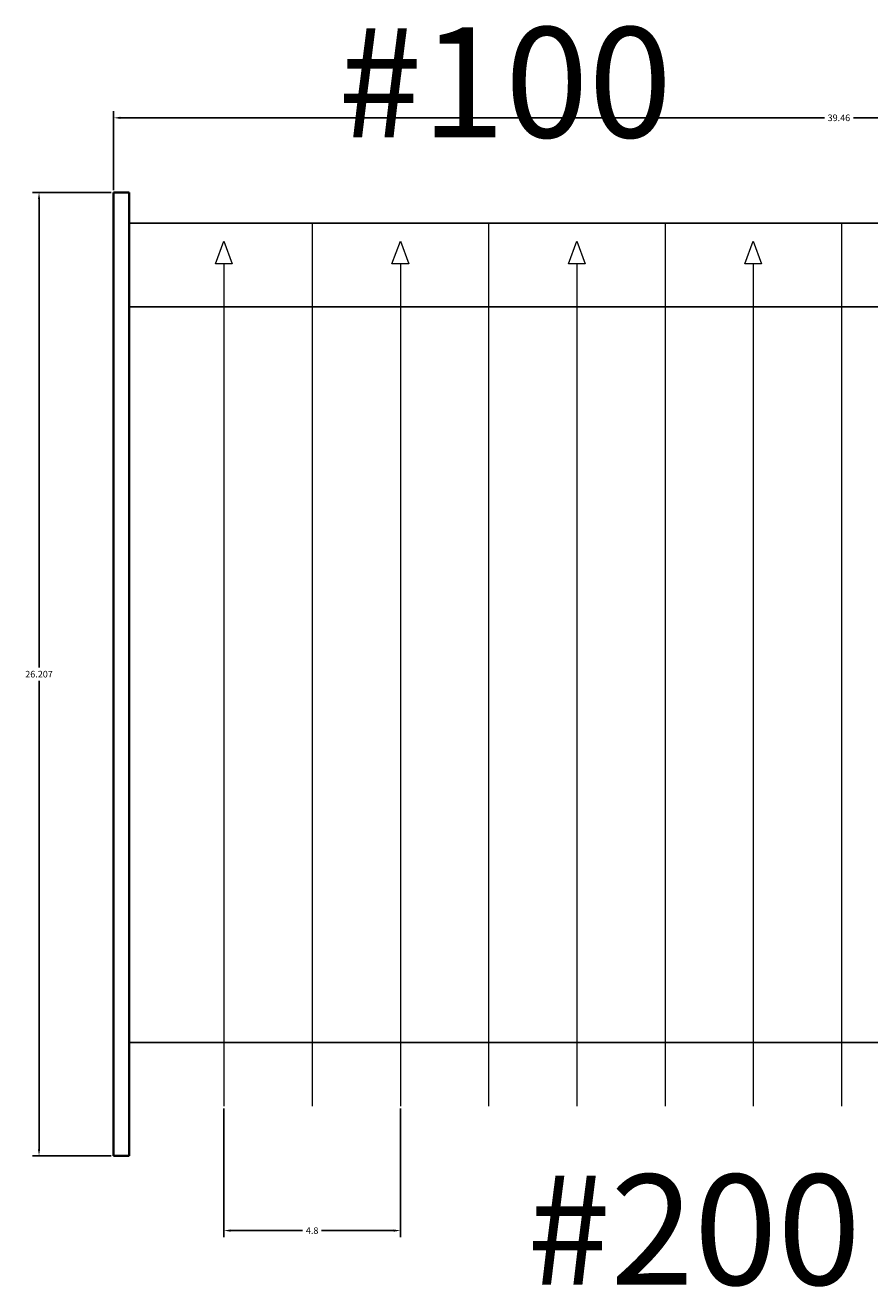
# Model space of a CAD drawing. Units: inches. Extents: x 756 to 915, y 488 to 695.
# Tile 15 of 25: x 768 to 791, y 626 to 660. Entities that reach past the tile are written whole.
import ezdxf

# ---------------------------------------------------------------- set-up
doc = ezdxf.new("R2010")
doc.units = ezdxf.units.IN
doc.header["$MEASUREMENT"] = 0
for name, color, linetype, lineweight in [('L-ANNO-TEXT', 7, 'Continuous', 25), ('L-FENC-PCKT', 7, 'Continuous', 18), ('L-FENC-POST', 7, 'Continuous', 35), ('L-FENC-RAIL', 7, 'Continuous', 25), ('M-DIMS', 2, 'Continuous', 18)]:
    doc.layers.add(name, color=color, linetype=linetype, lineweight=lineweight)
doc.styles.get("Standard").update_dxf_attribs({"font": 'arial.ttf'})
doc.dimstyles.get("Standard").update_dxf_attribs({"dimtxt": 0.18, "dimasz": 0.18, "dimexe": 0.18, "dimexo": 0.0625, "dimgap": 0.09, "dimtad": 0, "dimtih": 1, "dimtoh": 1, "dimdec": 0, "dimzin": 0, "dimdsep": 46, "dimlunit": 3, "dimtxsty": 'Standard', "dimcen": 0.09, "dimadec": 0, "dimazin": 0, "dimtfac": 1, "dimtdec": 0, "dimtofl": 0, "dimtmove": 0, "dimatfit": 3, "dimfxl": 1, "dimtolj": 1, "dimtzin": 0, "dimarcsym": 0})

# ---------------------------------------------------------------- blocks, each defined once
blk = doc.blocks.new('FENCE-POST-LEFT')
for p, q in [((0, 26.207), (0, 0)), ((0, 26.207), (0.426, 26.207)), ((0.426, 26.207), (0.426, 0)), ((0.426, 26.207), (0.426, 0)), ((0, 0), (0.426, 0))]:
    blk.add_line(p, q)
blk = doc.blocks.new('PICKET-SPEAR-LOW')
blk.add_line((0.228, 22.916), (0.228, 0))
blk.add_lwpolyline([(0.228, 22.916), (0, 22.916), (0.228, 23.528), (0.455, 22.916)], close=True)
blk = doc.blocks.new('*D32')
at = {"layer": 'Defpoints', "color": 0, "transparency": 16777216}
for p in [(809.674, 657.541), (770.216, 655.511), (809.674, 655.511)]:
    blk.add_point(p, dxfattribs=at)
at = {"layer": 'M-DIMS', "color": 0, "lineweight": -2, "transparency": 16777216}
for p, q in [((770.216, 655.574), (770.216, 657.721)), ((770.396, 657.541), (789.551, 657.541)), ((809.494, 657.541), (790.338, 657.541)), ((809.674, 655.574), (809.674, 657.721))]:
    blk.add_line(p, q, dxfattribs=at)
at = {"layer": 'M-DIMS', "color": 0, "transparency": 16777216}
for points in [[(770.396, 657.571), (770.396, 657.511), (770.216, 657.541)], [(809.494, 657.571), (809.494, 657.511), (809.674, 657.541)]]:
    blk.add_solid(points, dxfattribs=at)
at = {"layer": 'M-DIMS', "color": 0, "transparency": 16777216, "insert": (789.945, 657.541), "char_height": 0.18, "attachment_point": 5}
blk.add_mtext('\\A1;39.46', dxfattribs=at)
blk = doc.blocks.new('*D33')
at = {"layer": 'Defpoints', "color": 0, "transparency": 16777216}
for p in [(768.186, 655.511), (770.216, 655.511), (770.216, 629.304)]:
    blk.add_point(p, dxfattribs=at)
at = {"layer": 'M-DIMS', "color": 0, "lineweight": -2, "transparency": 16777216}
for p, q in [((770.153, 655.511), (768.006, 655.511)), ((768.186, 655.331), (768.186, 642.59)), ((768.186, 629.484), (768.186, 642.226)), ((770.153, 629.304), (768.006, 629.304))]:
    blk.add_line(p, q, dxfattribs=at)
at = {"layer": 'M-DIMS', "color": 0, "transparency": 16777216}
for points in [[(768.156, 655.331), (768.216, 655.331), (768.186, 655.511)], [(768.156, 629.484), (768.216, 629.484), (768.186, 629.304)]]:
    blk.add_solid(points, dxfattribs=at)
at = {"layer": 'M-DIMS', "color": 0, "transparency": 16777216, "insert": (768.186, 642.408), "char_height": 0.18, "attachment_point": 5}
blk.add_mtext('\\A1;26.207', dxfattribs=at)
blk = doc.blocks.new('*D34')
at = {"layer": 'Defpoints', "color": 0, "transparency": 16777216}
for p in [(773.215, 630.654), (778.015, 630.654), (778.015, 627.274)]:
    blk.add_point(p, dxfattribs=at)
at = {"layer": 'M-DIMS', "color": 0, "lineweight": -2, "transparency": 16777216}
for p, q in [((773.215, 630.591), (773.215, 627.094)), ((778.015, 630.591), (778.015, 627.094)), ((773.395, 627.274), (775.357, 627.274)), ((777.835, 627.274), (775.872, 627.274))]:
    blk.add_line(p, q, dxfattribs=at)
at = {"layer": 'M-DIMS', "color": 0, "transparency": 16777216}
for points in [[(773.395, 627.304), (773.395, 627.244), (773.215, 627.274)], [(777.835, 627.304), (777.835, 627.244), (778.015, 627.274)]]:
    blk.add_solid(points, dxfattribs=at)
at = {"layer": 'M-DIMS', "color": 0, "transparency": 16777216, "insert": (775.615, 627.274), "char_height": 0.18, "attachment_point": 5}
blk.add_mtext('\\A1;4.8', dxfattribs=at)

msp = doc.modelspace()

# ---------------------------------------------------------------- linework, layer by layer
at = {"layer": 'L-FENC-PCKT'}
for p, q in [((775.6147, 654.6726), (775.6147, 630.6539)), ((780.4145, 654.6726), (780.4145, 630.6539)), ((785.2143, 654.6726), (785.2143, 630.6539)), ((790.0141, 654.6726), (790.0141, 630.6539))]:
    msp.add_line(p, q, dxfattribs=at)
at = {"layer": 'L-FENC-RAIL'}
for p, q in [((770.6423, 654.6726), (809.2471, 654.6726)), ((770.6423, 652.3962), (809.2471, 652.3962)), ((770.6423, 632.386), (809.2471, 632.386))]:
    msp.add_line(p, q, dxfattribs=at)

# ---------------------------------------------------------------- block references
at = {"layer": 'L-FENC-PCKT'}
for p in [(772.987, 630.6543), (777.7868, 630.6543), (782.5866, 630.6543), (787.3865, 630.6543)]:
    msp.add_blockref('PICKET-SPEAR-LOW', p, dxfattribs=at)
at = {"layer": 'L-FENC-POST'}
msp.add_blockref('FENCE-POST-LEFT', (770.216, 629.3043), dxfattribs=at)

# ---------------------------------------------------------------- texts
at = {"layer": 'L-ANNO-TEXT'}
for s, p in [('#100', (776.3182, 657.006)), ('#200', (781.4569, 625.7989))]:
    msp.add_text(s, height=3, dxfattribs=at).set_placement(p)

# ---------------------------------------------------------------- dimensions: what is measured, and where the dimension line sits
at = {"layer": 'M-DIMS'}
for base, p1, p2, override, picture, middle in [((809.6738, 657.5412), (770.2156, 655.5112), (809.6738, 655.5112), {"dimdec": 2, "dimlfac": 1, "dimrnd": 0, "dimzin": 0, "dimdsep": 46, "dimlunit": 2}, '*D32', (789.9447, 657.5412)), ((778.0146, 627.2744), (773.2147, 630.6539), (778.0146, 630.6539), {"dimdec": 1, "dimlfac": 1, "dimrnd": 0, "dimzin": 0, "dimdsep": 46, "dimlunit": 2}, '*D34', (775.6147, 627.2744))]:
    dim = msp.add_linear_dim(base=base, p1=p1, p2=p2, dimstyle='Standard', override=override, dxfattribs=at)
    dim.commit()
    dim.dimension.update_dxf_attribs({"geometry": picture, "text_midpoint": middle})
dim = msp.add_linear_dim(base=(768.1856, 655.5112), p1=(770.2156, 629.3044), p2=(770.2156, 655.5112), angle=90, dimstyle='Standard', override={"dimdec": 3, "dimlfac": 1, "dimrnd": 0, "dimzin": 0, "dimdsep": 46, "dimlunit": 2}, dxfattribs=at)
dim.commit()
dim.dimension.update_dxf_attribs({"geometry": '*D33', "text_midpoint": (768.1856, 642.4078)})

doc.saveas('drawing.dxf')
